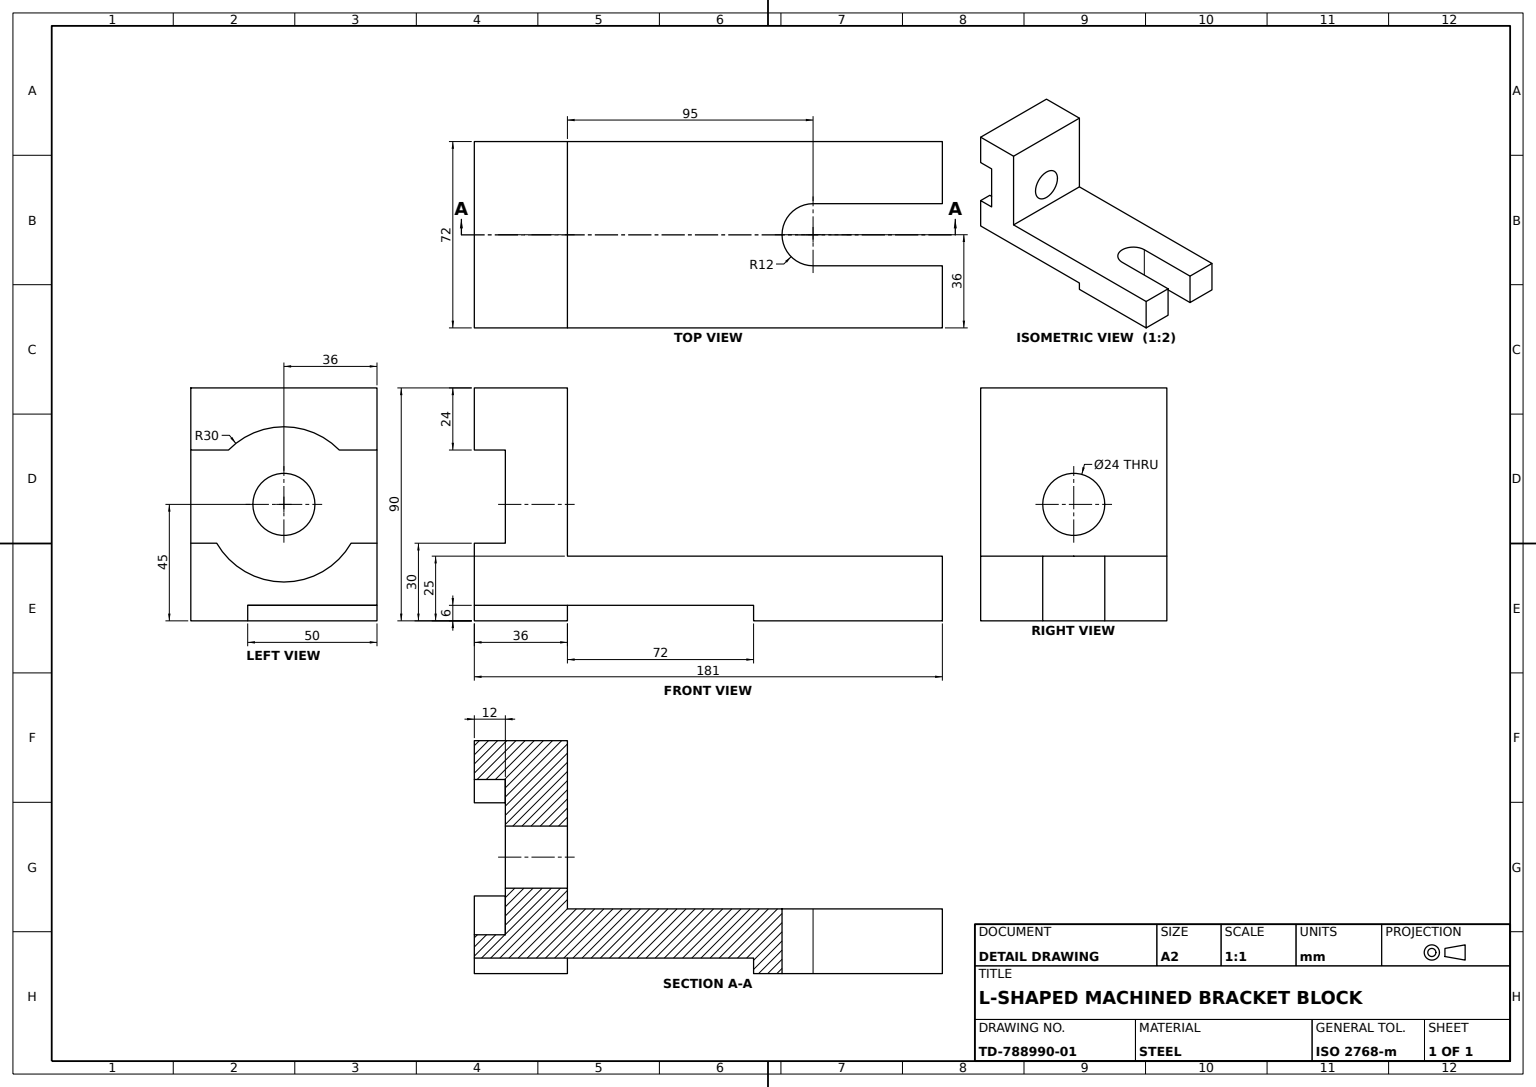
SolidWorks part; units mm, degrees
material "Plain Carbon Steel"
ref_plane "Front Plane" through (0, 0, 0) normal (0, 0, 1) x (1, 0, 0)
ref_plane "Top Plane" through (0, 0, 0) normal (0, 1, 0) x (1, 0, 0)
ref_plane "Right Plane" through (0, 0, 0) normal (1, 0, 0) x (0, 0, -1)
sketch "Base Block Sketch" plane through (0, 0, 0) normal (0, 0, 1) x (1, 0, 0)
  line L1 (0, 0) -> (72, 0)
  line L2 (0, 0) -> (0, 90)
  line L3 (0, 90) -> (72, 90)
  line L4 (72, 0) -> (72, 90)
  dimension "D1" = 90
  dimension "D2" = 72
extrude "Base Block 90x72x36" add sketch "Base Block Sketch" along normal mid plane 36
sketch "Bore Sketch" plane through (72, 0, 0) normal (1, 0, 0) x (0, 0, -1)
  line L0 (-18, 45) -> (18, 45) construction
  line L1 (-18, 0) -> (-18, 90) construction
  line L2 (18, 0) -> (18, 90) construction
  line L3 (0, 90) -> (0, 0) construction
  line L4 (-18, 90) -> (18, 90) construction
  line L5 (-18, 66) -> (-6, 66)
  line L6 (-6, 66) -> (-6, 45)
  line L7 (-6, 45) -> (-6, 30)
  line L8 (-6, 30) -> (-18, 30)
  line L9 (-18, 30) -> (-18, 66)
  line L10 (-18, 0) -> (18, 0) construction
  dimension "D1" = 24
  dimension "D2" = 30
  dimension "D3" = 12
sketch "Arc Recess Sketch" plane through (0, 0, 18) normal (0, 0, 1) x (1, 0, 0)
  line L0 (72, 45.1913) -> (0, 45) construction
  line L1 (72, 30) -> (72, 66) construction
  line L2 (0, 90) -> (0, 0) construction
  line L3 (36, 90) -> (36, 0) construction
  line L4 (72, 90) -> (0, 90) construction
  line L5 (0, 0) -> (72, 0) construction
  circle A0 centre (36, 45) radius 30
  dimension "D1" = 60
  dimension "D2" = 0.1913
extrude "Arc Recess Ø60" cut sketch "Arc Recess Sketch" against normal blind 12
extrude "Bore Ø24" cut sketch "Bore Sketch" against normal through all
sketch "Recess Relief Sketch" plane through (0, 0, 6) normal (0, 0, 1) x (1, 0, 0)
  line L6 (61.9808, 30) -> (72, 30)
  line L7 (72, 30) -> (72, 66)
  line L8 (72, 66) -> (57.4243, 66)
  line L9 (14.5757, 66) -> (0, 66)
  line L10 (0, 66) -> (0, 30)
  line L11 (0, 30) -> (10.0192, 30)
  line L12 (61.9808, 30) -> (72, 30)
  line L13 (72, 30) -> (72, 66)
  line L14 (72, 66) -> (57.4243, 66)
  line L15 (14.5757, 66) -> (0, 66)
  line L16 (0, 66) -> (0, 30)
  line L17 (0, 30) -> (10.0192, 30)
  circle A0 centre (36, 45) radius 12
  arc A2 (10.0192, 30) -> (61.9808, 30) centre (36, 45) ccw
  arc A3 (57.4243, 66) -> (14.5757, 66) centre (36, 45) ccw
  arc A4 (10.0192, 30) -> (61.9808, 30) centre (36, 45) ccw
  arc A5 (57.4243, 66) -> (14.5757, 66) centre (36, 45) ccw
  dimension "D2" = 24
  dimension "D1" = 0
extrude "Recess Relief Cut" cut sketch "Recess Relief Sketch" against normal through all contours A0
sketch "Bottom Groove Sketch" plane through (0, 0, 18) normal (0, 0, 1) x (1, 0, 0)
  line L0 (22, 0) -> (22, 6)
  line L1 (0, 0) -> (72, 0) construction
  line L2 (22, 6) -> (72, 6)
  line L3 (72, 0) -> (72, 30) construction
  line L4 (22, 0) -> (72, 0)
  line L5 (72, 0) -> (72, 6)
  dimension "D1" = 6
  dimension "D2" = 50
extrude "Bottom Groove 6x50" cut sketch "Bottom Groove Sketch" against normal through all
sketch "Fork Arm Sketch" plane through (72, 0, 0) normal (1, 0, 0) x (0, 0, -1)
  line L0 (18, 6) -> (90, 6)
  line L1 (90, 6) -> (90, 0)
  line L2 (90, 0) -> (163, 0)
  line L3 (163, 0) -> (163, 25)
  line L4 (163, 25) -> (18, 25)
  line L5 (18, 6) -> (18, 90) construction
  line L6 (18, 25) -> (18, 6)
  dimension "D1" = 72
  dimension "D2" = 145
  dimension "D3" = 25
extrude "Fork Arm" add sketch "Fork Arm Sketch" against normal blind 72
sketch "Fork Slot Sketch" plane through (0, 25, 0) normal (0, 1, 0) x (1, 0, 0)
  line L0 (72, 163) -> (72, 18) construction
  line L4 (48, 163) -> (48, 113)
  line L5 (24, 163) -> (24, 113)
  line L6 (24, 163) -> (48, 163)
  arc A0 (24, 113) -> (48, 113) centre (36, 113) ccw
  dimension "D4" = 24
  dimension "D1" = 50
  dimension "D2" = 36
  dimension "D3" = 95
extrude "Fork Slot 24" cut sketch "Fork Slot Sketch" against normal through all
